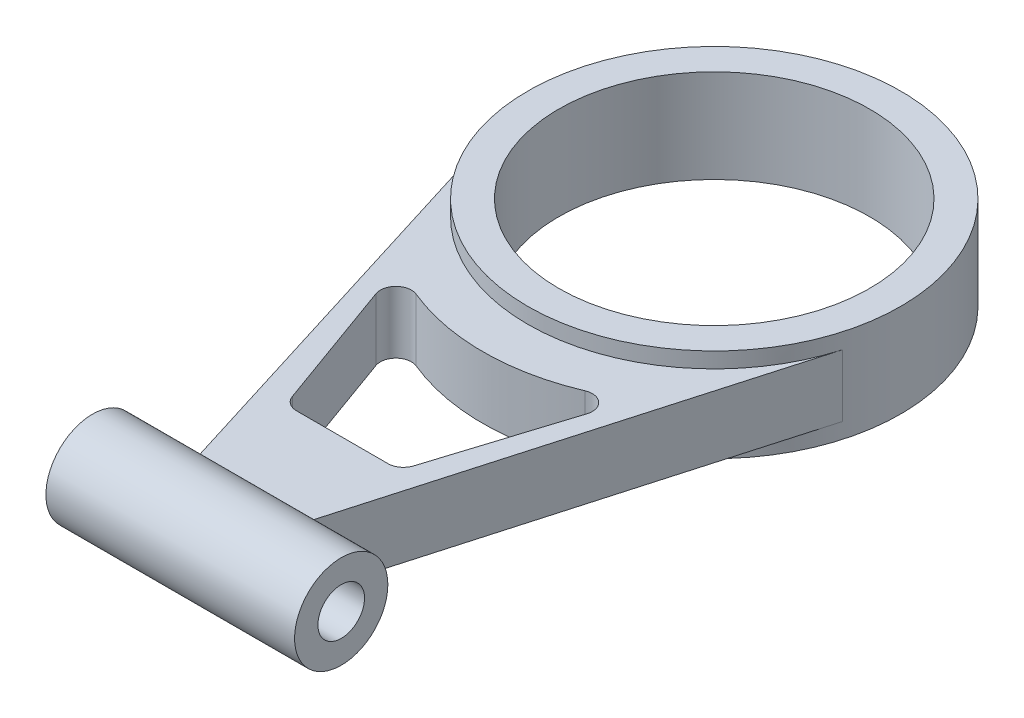
ISO-10303-21;
HEADER;
FILE_DESCRIPTION(('STEP AP214'),'2;1');
FILE_NAME('part.step','',(''),(''),'','','');
FILE_SCHEMA(('AUTOMOTIVE_DESIGN { 1 0 10303 214 1 1 1 1 }'));
ENDSEC;
DATA;
#1=APPLICATION_CONTEXT('core data for automotive mechanical design processes');
#2=APPLICATION_PROTOCOL_DEFINITION('international standard','automotive_design',2000,#1);
#3=PRODUCT_CONTEXT('',#1,'mechanical');
#4=PRODUCT('Part','Part','',(#3));
#5=PRODUCT_RELATED_PRODUCT_CATEGORY('part','',(#4));
#6=PRODUCT_DEFINITION_FORMATION('','',#4);
#7=PRODUCT_DEFINITION_CONTEXT('part definition',#1,'design');
#8=PRODUCT_DEFINITION('design','',#6,#7);
#9=PRODUCT_DEFINITION_SHAPE('','',#8);
#10=(LENGTH_UNIT() NAMED_UNIT(*) SI_UNIT(.MILLI.,.METRE.));
#11=(NAMED_UNIT(*) PLANE_ANGLE_UNIT() SI_UNIT($,.RADIAN.));
#12=(NAMED_UNIT(*) SI_UNIT($,.STERADIAN.) SOLID_ANGLE_UNIT());
#13=UNCERTAINTY_MEASURE_WITH_UNIT(LENGTH_MEASURE(1.E-05),#10,'distance_accuracy_value','');
#14=(GEOMETRIC_REPRESENTATION_CONTEXT(3) GLOBAL_UNCERTAINTY_ASSIGNED_CONTEXT((#13)) GLOBAL_UNIT_ASSIGNED_CONTEXT((#10,
#11,#12)) REPRESENTATION_CONTEXT('',''));
#15=CARTESIAN_POINT('',(0.,0.,0.));
#16=DIRECTION('',(0.,0.,1.));
#17=DIRECTION('',(1.,0.,0.));
#18=AXIS2_PLACEMENT_3D('',#15,#16,#17);
#19=CARTESIAN_POINT('',(40.,0.,0.));
#20=DIRECTION('',(1.,0.,0.));
#21=DIRECTION('',(0.,0.,-1.));
#22=AXIS2_PLACEMENT_3D('',#19,#20,#21);
#23=PLANE('',#22);
#24=CARTESIAN_POINT('',(40.,0.,0.));
#25=DIRECTION('',(1.,0.,0.));
#26=DIRECTION('',(0.,0.,-1.));
#27=AXIS2_PLACEMENT_3D('',#24,#25,#26);
#28=CIRCLE('',#27,15.);
#29=CARTESIAN_POINT('',(40.,0.,-15.));
#30=VERTEX_POINT('',#29);
#31=EDGE_CURVE('E219',#30,#30,#28,.T.);
#32=ORIENTED_EDGE('',*,*,#31,.T.);
#33=EDGE_LOOP('',(#32));
#34=FACE_BOUND('',#33,.T.);
#35=CARTESIAN_POINT('',(40.,0.,0.));
#36=DIRECTION('',(1.,0.,0.));
#37=DIRECTION('',(0.,0.,-1.));
#38=AXIS2_PLACEMENT_3D('',#35,#36,#37);
#39=CIRCLE('',#38,7.5);
#40=CARTESIAN_POINT('',(40.,0.,-7.5));
#41=VERTEX_POINT('',#40);
#42=EDGE_CURVE('E212',#41,#41,#39,.T.);
#43=ORIENTED_EDGE('',*,*,#42,.F.);
#44=EDGE_LOOP('',(#43));
#45=FACE_BOUND('',#44,.T.);
#46=ADVANCED_FACE('F43',(#34,#45),#23,.T.);
#47=CARTESIAN_POINT('',(-40.,0.,0.));
#48=DIRECTION('',(1.,0.,0.));
#49=DIRECTION('',(0.,0.,-1.));
#50=AXIS2_PLACEMENT_3D('',#47,#48,#49);
#51=PLANE('',#50);
#52=CARTESIAN_POINT('',(-40.,0.,0.));
#53=DIRECTION('',(1.,0.,0.));
#54=DIRECTION('',(0.,0.,-1.));
#55=AXIS2_PLACEMENT_3D('',#52,#53,#54);
#56=CIRCLE('',#55,15.);
#57=CARTESIAN_POINT('',(-40.,0.,-15.));
#58=VERTEX_POINT('',#57);
#59=EDGE_CURVE('E220',#58,#58,#56,.T.);
#60=ORIENTED_EDGE('',*,*,#59,.F.);
#61=EDGE_LOOP('',(#60));
#62=FACE_BOUND('',#61,.T.);
#63=CARTESIAN_POINT('',(-40.,0.,0.));
#64=DIRECTION('',(1.,0.,0.));
#65=DIRECTION('',(0.,0.,-1.));
#66=AXIS2_PLACEMENT_3D('',#63,#64,#65);
#67=CIRCLE('',#66,7.5);
#68=CARTESIAN_POINT('',(-40.,0.,-7.5));
#69=VERTEX_POINT('',#68);
#70=EDGE_CURVE('E213',#69,#69,#67,.T.);
#71=ORIENTED_EDGE('',*,*,#70,.T.);
#72=EDGE_LOOP('',(#71));
#73=FACE_BOUND('',#72,.T.);
#74=ADVANCED_FACE('F286',(#62,#73),#51,.F.);
#75=CARTESIAN_POINT('',(40.,0.,0.));
#76=DIRECTION('',(-1.,0.,0.));
#77=DIRECTION('',(0.,0.,1.));
#78=AXIS2_PLACEMENT_3D('',#75,#76,#77);
#79=CYLINDRICAL_SURFACE('',#78,15.);
#80=CARTESIAN_POINT('',(16.801488358698,0.,0.));
#81=DIRECTION('',(-0.961726920405214,0.,-0.274009727141033));
#82=DIRECTION('',(-0.274009727141033,0.,0.961726920405214));
#83=AXIS2_PLACEMENT_3D('',#80,#81,#82);
#84=ELLIPSE('',#83,15.596943042501,15.);
#85=CARTESIAN_POINT('',(19.986926778813,10.,-11.1803398874989));
#86=VERTEX_POINT('',#85);
#87=CARTESIAN_POINT('',(19.986926778813,-10.,-11.1803398874989));
#88=VERTEX_POINT('',#87);
#89=EDGE_CURVE('E226',#86,#88,#84,.T.);
#90=ORIENTED_EDGE('',*,*,#89,.F.);
#91=DIRECTION('',(-1.,0.,0.));
#92=VECTOR('',#91,1.);
#93=CARTESIAN_POINT('',(40.,10.,-11.1803398874989));
#94=LINE('',#93,#92);
#95=CARTESIAN_POINT('',(-16.5703284007776,10.,-11.1803398874989));
#96=VERTEX_POINT('',#95);
#97=EDGE_CURVE('E233',#86,#96,#94,.T.);
#98=ORIENTED_EDGE('',*,*,#97,.T.);
#99=CARTESIAN_POINT('',(-13.0948278450043,0.,0.));
#100=DIRECTION('',(-0.9549252516487,0.,0.29684636390508));
#101=DIRECTION('',(-0.29684636390508,0.,-0.9549252516487));
#102=AXIS2_PLACEMENT_3D('',#99,#100,#101);
#103=ELLIPSE('',#102,15.7080357589269,15.);
#104=CARTESIAN_POINT('',(-16.5703284007776,-10.,-11.1803398874989));
#105=VERTEX_POINT('',#104);
#106=EDGE_CURVE('E231',#96,#105,#103,.T.);
#107=ORIENTED_EDGE('',*,*,#106,.T.);
#108=DIRECTION('',(-1.,0.,0.));
#109=VECTOR('',#108,1.);
#110=CARTESIAN_POINT('',(40.,-10.,-11.1803398874989));
#111=LINE('',#110,#109);
#112=EDGE_CURVE('E224',#88,#105,#111,.T.);
#113=ORIENTED_EDGE('',*,*,#112,.F.);
#114=EDGE_LOOP('',(#90,#98,#107,#113));
#115=FACE_BOUND('',#114,.T.);
#116=ORIENTED_EDGE('',*,*,#31,.F.);
#117=EDGE_LOOP('',(#116));
#118=FACE_BOUND('',#117,.T.);
#119=ORIENTED_EDGE('',*,*,#59,.T.);
#120=EDGE_LOOP('',(#119));
#121=FACE_BOUND('',#120,.T.);
#122=ADVANCED_FACE('F44',(#115,#118,#121),#79,.T.);
#123=CARTESIAN_POINT('',(40.,0.,0.));
#124=DIRECTION('',(-1.,0.,0.));
#125=DIRECTION('',(0.,0.,1.));
#126=AXIS2_PLACEMENT_3D('',#123,#124,#125);
#127=CYLINDRICAL_SURFACE('',#126,7.5);
#128=ORIENTED_EDGE('',*,*,#42,.T.);
#129=EDGE_LOOP('',(#128));
#130=FACE_BOUND('',#129,.T.);
#131=ORIENTED_EDGE('',*,*,#70,.F.);
#132=EDGE_LOOP('',(#131));
#133=FACE_BOUND('',#132,.T.);
#134=ADVANCED_FACE('F293',(#130,#133),#127,.F.);
#135=CARTESIAN_POINT('',(0.,10.,0.));
#136=DIRECTION('',(0.,1.,0.));
#137=DIRECTION('',(0.,0.,1.));
#138=AXIS2_PLACEMENT_3D('',#135,#136,#137);
#139=PLANE('',#138);
#140=CARTESIAN_POINT('',(-13.0584068998663,10.,-43.7136049203832));
#141=DIRECTION('',(0.,1.,0.));
#142=DIRECTION('',(0.,0.,-1.));
#143=AXIS2_PLACEMENT_3D('',#140,#141,#142);
#144=CIRCLE('',#143,5.);
#145=CARTESIAN_POINT('',(-17.7618405284644,10.,-42.0172228580598));
#146=VERTEX_POINT('',#145);
#147=CARTESIAN_POINT('',(-13.0584068998663,10.,-38.7136049203832));
#148=VERTEX_POINT('',#147);
#149=EDGE_CURVE('E59',#146,#148,#144,.T.);
#150=ORIENTED_EDGE('',*,*,#149,.F.);
#151=DIRECTION('',(0.339276412464669,0.,0.940686725719622));
#152=VECTOR('',#151,1.);
#153=CARTESIAN_POINT('',(-32.9546293939201,10.,-84.1411498017971));
#154=LINE('',#153,#152);
#155=CARTESIAN_POINT('',(-32.9546293939206,10.,-84.1411498017969));
#156=VERTEX_POINT('',#155);
#157=EDGE_CURVE('E167',#156,#146,#154,.T.);
#158=ORIENTED_EDGE('',*,*,#157,.F.);
#159=CARTESIAN_POINT('',(-28.2511957653232,10.,-85.8375318641209));
#160=DIRECTION('',(0.,1.,0.));
#161=DIRECTION('',(0.,0.,1.));
#162=AXIS2_PLACEMENT_3D('',#159,#160,#161);
#163=CIRCLE('',#162,4.99999999999952);
#164=CARTESIAN_POINT('',(-26.341109619655,10.,-90.4583078721229));
#165=VERTEX_POINT('',#164);
#166=EDGE_CURVE('E162',#165,#156,#163,.T.);
#167=ORIENTED_EDGE('',*,*,#166,.F.);
#168=CARTESIAN_POINT('',(0.400096419681878,10.,-155.149171984157));
#169=DIRECTION('',(0.,-1.,0.));
#170=DIRECTION('',(0.,0.,1.));
#171=AXIS2_PLACEMENT_3D('',#168,#169,#170);
#172=CIRCLE('',#171,70.);
#173=CARTESIAN_POINT('',(27.7252493420679,10.,-90.702791032484));
#174=VERTEX_POINT('',#173);
#175=EDGE_CURVE('E159',#174,#165,#172,.T.);
#176=ORIENTED_EDGE('',*,*,#175,.F.);
#177=CARTESIAN_POINT('',(29.6770459793811,10.,-86.0994781073645));
#178=DIRECTION('',(0.,1.,0.));
#179=DIRECTION('',(0.,0.,1.));
#180=AXIS2_PLACEMENT_3D('',#177,#178,#179);
#181=CIRCLE('',#180,5.);
#182=CARTESIAN_POINT('',(34.4458674515617,10.,-84.5967000909994));
#183=VERTEX_POINT('',#182);
#184=EDGE_CURVE('E152',#183,#174,#181,.T.);
#185=ORIENTED_EDGE('',*,*,#184,.F.);
#186=DIRECTION('',(0.300555603273013,0.,-0.953764294436102));
#187=VECTOR('',#186,1.);
#188=CARTESIAN_POINT('',(21.088991166422,10.,-42.2108269040181));
#189=LINE('',#188,#187);
#190=CARTESIAN_POINT('',(21.088991166422,10.,-42.2108269040181));
#191=VERTEX_POINT('',#190);
#192=EDGE_CURVE('E155',#191,#183,#189,.T.);
#193=ORIENTED_EDGE('',*,*,#192,.F.);
#194=CARTESIAN_POINT('',(16.3201696942414,10.,-43.7136049203832));
#195=DIRECTION('',(0.,1.,0.));
#196=DIRECTION('',(0.,0.,1.));
#197=AXIS2_PLACEMENT_3D('',#194,#195,#196);
#198=CIRCLE('',#197,5.);
#199=CARTESIAN_POINT('',(16.3201696942414,10.,-38.7136049203832));
#200=VERTEX_POINT('',#199);
#201=EDGE_CURVE('E134',#200,#191,#198,.T.);
#202=ORIENTED_EDGE('',*,*,#201,.F.);
#203=DIRECTION('',(1.,0.,0.));
#204=VECTOR('',#203,1.);
#205=CARTESIAN_POINT('',(-13.0584068998663,10.,-38.7136049203832));
#206=LINE('',#205,#204);
#207=EDGE_CURVE('E145',#148,#200,#206,.T.);
#208=ORIENTED_EDGE('',*,*,#207,.F.);
#209=EDGE_LOOP('',(#150,#158,#167,#176,#185,#193,#202,#208));
#210=FACE_BOUND('',#209,.T.);
#211=ORIENTED_EDGE('',*,*,#97,.F.);
#212=DIRECTION('',(0.274009727141033,0.,-0.961726920405214));
#213=VECTOR('',#212,1.);
#214=CARTESIAN_POINT('',(15.5400102572058,10.,4.42757073759744));
#215=LINE('',#214,#213);
#216=CARTESIAN_POINT('',(57.7036152243128,10.,-143.559416371538));
#217=VERTEX_POINT('',#216);
#218=EDGE_CURVE('E199',#86,#217,#215,.T.);
#219=ORIENTED_EDGE('',*,*,#218,.T.);
#220=CARTESIAN_POINT('',(0.,10.,-160.));
#221=DIRECTION('',(0.,1.,0.));
#222=DIRECTION('',(0.,0.,1.));
#223=AXIS2_PLACEMENT_3D('',#220,#221,#222);
#224=CIRCLE('',#223,60.);
#225=CARTESIAN_POINT('',(-57.295515098922,10.,-142.189218165695));
#226=VERTEX_POINT('',#225);
#227=EDGE_CURVE('E192',#226,#217,#224,.T.);
#228=ORIENTED_EDGE('',*,*,#227,.F.);
#229=DIRECTION('',(-0.29684636390508,0.,-0.9549252516487));
#230=VECTOR('',#229,1.);
#231=CARTESIAN_POINT('',(-11.9409408984323,10.,3.71193963211804));
#232=LINE('',#231,#230);
#233=EDGE_CURVE('E197',#96,#226,#232,.T.);
#234=ORIENTED_EDGE('',*,*,#233,.F.);
#235=EDGE_LOOP('',(#211,#219,#228,#234));
#236=FACE_BOUND('',#235,.T.);
#237=ADVANCED_FACE('F146',(#210,#236),#139,.T.);
#238=CARTESIAN_POINT('',(0.,-10.,0.));
#239=DIRECTION('',(0.,1.,0.));
#240=DIRECTION('',(0.,0.,1.));
#241=AXIS2_PLACEMENT_3D('',#238,#239,#240);
#242=PLANE('',#241);
#243=DIRECTION('',(0.339276412464669,0.,0.940686725719622));
#244=VECTOR('',#243,1.);
#245=CARTESIAN_POINT('',(-2.30738693020975,-10.,0.832202622239151));
#246=LINE('',#245,#244);
#247=CARTESIAN_POINT('',(-32.9546293939206,-10.,-84.1411498017969));
#248=VERTEX_POINT('',#247);
#249=CARTESIAN_POINT('',(-17.7618405284644,-10.,-42.0172228580598));
#250=VERTEX_POINT('',#249);
#251=EDGE_CURVE('E51',#248,#250,#246,.T.);
#252=ORIENTED_EDGE('',*,*,#251,.T.);
#253=CARTESIAN_POINT('',(-13.0584068998663,-10.,-43.7136049203832));
#254=DIRECTION('',(0.,1.,0.));
#255=DIRECTION('',(0.,0.,1.));
#256=AXIS2_PLACEMENT_3D('',#253,#254,#255);
#257=CIRCLE('',#256,5.);
#258=CARTESIAN_POINT('',(-13.0584068998663,-10.,-38.7136049203832));
#259=VERTEX_POINT('',#258);
#260=EDGE_CURVE('E11',#250,#259,#257,.T.);
#261=ORIENTED_EDGE('',*,*,#260,.T.);
#262=DIRECTION('',(1.,0.,0.));
#263=VECTOR('',#262,1.);
#264=CARTESIAN_POINT('',(0.,-10.,-38.7136049203832));
#265=LINE('',#264,#263);
#266=CARTESIAN_POINT('',(16.3201696942414,-10.,-38.7136049203832));
#267=VERTEX_POINT('',#266);
#268=EDGE_CURVE('E234',#259,#267,#265,.T.);
#269=ORIENTED_EDGE('',*,*,#268,.T.);
#270=CARTESIAN_POINT('',(16.3201696942414,-10.,-43.7136049203832));
#271=DIRECTION('',(0.,1.,0.));
#272=DIRECTION('',(0.,0.,1.));
#273=AXIS2_PLACEMENT_3D('',#270,#271,#272);
#274=CIRCLE('',#273,5.);
#275=CARTESIAN_POINT('',(21.088991166422,-10.,-42.2108269040181));
#276=VERTEX_POINT('',#275);
#277=EDGE_CURVE('E138',#267,#276,#274,.T.);
#278=ORIENTED_EDGE('',*,*,#277,.T.);
#279=DIRECTION('',(0.300555603273013,0.,-0.953764294436102));
#280=VECTOR('',#279,1.);
#281=CARTESIAN_POINT('',(7.08382319004432,-10.,2.23229446183233));
#282=LINE('',#281,#280);
#283=CARTESIAN_POINT('',(34.4458674515617,-10.,-84.5967000909994));
#284=VERTEX_POINT('',#283);
#285=EDGE_CURVE('E236',#276,#284,#282,.T.);
#286=ORIENTED_EDGE('',*,*,#285,.T.);
#287=CARTESIAN_POINT('',(29.6770459793811,-10.,-86.0994781073645));
#288=DIRECTION('',(0.,1.,0.));
#289=DIRECTION('',(0.,0.,1.));
#290=AXIS2_PLACEMENT_3D('',#287,#288,#289);
#291=CIRCLE('',#290,5.);
#292=CARTESIAN_POINT('',(27.7252493420679,-10.,-90.702791032484));
#293=VERTEX_POINT('',#292);
#294=EDGE_CURVE('E243',#284,#293,#291,.T.);
#295=ORIENTED_EDGE('',*,*,#294,.T.);
#296=CARTESIAN_POINT('',(0.400096419681878,-10.,-155.149171984157));
#297=DIRECTION('',(0.,1.,0.));
#298=DIRECTION('',(0.,0.,1.));
#299=AXIS2_PLACEMENT_3D('',#296,#297,#298);
#300=CIRCLE('',#299,70.);
#301=CARTESIAN_POINT('',(-26.341109619655,-10.,-90.4583078721229));
#302=VERTEX_POINT('',#301);
#303=EDGE_CURVE('E242',#293,#302,#300,.F.);
#304=ORIENTED_EDGE('',*,*,#303,.T.);
#305=CARTESIAN_POINT('',(-28.2511957653232,-10.,-85.8375318641209));
#306=DIRECTION('',(0.,1.,0.));
#307=DIRECTION('',(0.,0.,1.));
#308=AXIS2_PLACEMENT_3D('',#305,#306,#307);
#309=CIRCLE('',#308,4.99999999999952);
#310=EDGE_CURVE('E250',#302,#248,#309,.T.);
#311=ORIENTED_EDGE('',*,*,#310,.T.);
#312=EDGE_LOOP('',(#252,#261,#269,#278,#286,#295,#304,#311));
#313=FACE_BOUND('',#312,.T.);
#314=DIRECTION('',(0.274009727141033,0.,-0.961726920405214));
#315=VECTOR('',#314,1.);
#316=CARTESIAN_POINT('',(15.5400102572058,-10.,4.42757073759744));
#317=LINE('',#316,#315);
#318=CARTESIAN_POINT('',(57.7036152243128,-10.,-143.559416371538));
#319=VERTEX_POINT('',#318);
#320=EDGE_CURVE('E196',#88,#319,#317,.T.);
#321=ORIENTED_EDGE('',*,*,#320,.F.);
#322=ORIENTED_EDGE('',*,*,#112,.T.);
#323=DIRECTION('',(-0.29684636390508,0.,-0.9549252516487));
#324=VECTOR('',#323,1.);
#325=CARTESIAN_POINT('',(-11.9409408984323,-10.,3.71193963211804));
#326=LINE('',#325,#324);
#327=CARTESIAN_POINT('',(-57.295515098922,-10.,-142.189218165695));
#328=VERTEX_POINT('',#327);
#329=EDGE_CURVE('E204',#105,#328,#326,.T.);
#330=ORIENTED_EDGE('',*,*,#329,.T.);
#331=CARTESIAN_POINT('',(0.,-10.,-160.));
#332=DIRECTION('',(0.,1.,0.));
#333=DIRECTION('',(0.,0.,1.));
#334=AXIS2_PLACEMENT_3D('',#331,#332,#333);
#335=CIRCLE('',#334,60.);
#336=EDGE_CURVE('E191',#328,#319,#335,.T.);
#337=ORIENTED_EDGE('',*,*,#336,.T.);
#338=EDGE_LOOP('',(#321,#322,#330,#337));
#339=FACE_BOUND('',#338,.T.);
#340=ADVANCED_FACE('F253',(#313,#339),#242,.F.);
#341=CARTESIAN_POINT('',(-11.9409408984323,10.,3.71193963211804));
#342=DIRECTION('',(-0.9549252516487,0.,0.29684636390508));
#343=DIRECTION('',(0.29684636390508,0.,0.9549252516487));
#344=AXIS2_PLACEMENT_3D('',#341,#342,#343);
#345=PLANE('',#344);
#346=ORIENTED_EDGE('',*,*,#106,.F.);
#347=ORIENTED_EDGE('',*,*,#233,.T.);
#348=DIRECTION('',(0.,-1.,0.));
#349=VECTOR('',#348,1.);
#350=CARTESIAN_POINT('',(-57.295515098922,10.,-142.189218165695));
#351=LINE('',#350,#349);
#352=EDGE_CURVE('E209',#226,#328,#351,.T.);
#353=ORIENTED_EDGE('',*,*,#352,.T.);
#354=ORIENTED_EDGE('',*,*,#329,.F.);
#355=EDGE_LOOP('',(#346,#347,#353,#354));
#356=FACE_BOUND('',#355,.T.);
#357=ADVANCED_FACE('F297',(#356),#345,.T.);
#358=CARTESIAN_POINT('',(15.5400102572058,10.,4.42757073759744));
#359=DIRECTION('',(-0.961726920405214,0.,-0.274009727141033));
#360=DIRECTION('',(-0.274009727141033,0.,0.961726920405214));
#361=AXIS2_PLACEMENT_3D('',#358,#359,#360);
#362=PLANE('',#361);
#363=ORIENTED_EDGE('',*,*,#218,.F.);
#364=ORIENTED_EDGE('',*,*,#89,.T.);
#365=ORIENTED_EDGE('',*,*,#320,.T.);
#366=DIRECTION('',(0.,-1.,0.));
#367=VECTOR('',#366,1.);
#368=CARTESIAN_POINT('',(57.7036152243128,10.,-143.559416371538));
#369=LINE('',#368,#367);
#370=EDGE_CURVE('E205',#217,#319,#369,.T.);
#371=ORIENTED_EDGE('',*,*,#370,.F.);
#372=EDGE_LOOP('',(#363,#364,#365,#371));
#373=FACE_BOUND('',#372,.T.);
#374=ADVANCED_FACE('F305',(#373),#362,.F.);
#375=CARTESIAN_POINT('',(0.,15.,-160.));
#376=DIRECTION('',(0.,-1.,0.));
#377=DIRECTION('',(0.,0.,-1.));
#378=AXIS2_PLACEMENT_3D('',#375,#376,#377);
#379=CYLINDRICAL_SURFACE('',#378,60.);
#380=CARTESIAN_POINT('',(0.,15.,-160.));
#381=DIRECTION('',(0.,1.,0.));
#382=DIRECTION('',(0.,0.,1.));
#383=AXIS2_PLACEMENT_3D('',#380,#381,#382);
#384=CIRCLE('',#383,60.);
#385=CARTESIAN_POINT('',(0.,15.,-100.));
#386=VERTEX_POINT('',#385);
#387=EDGE_CURVE('E186',#386,#386,#384,.T.);
#388=ORIENTED_EDGE('',*,*,#387,.F.);
#389=EDGE_LOOP('',(#388));
#390=FACE_BOUND('',#389,.T.);
#391=CARTESIAN_POINT('',(0.,-15.,-160.));
#392=DIRECTION('',(0.,1.,0.));
#393=DIRECTION('',(0.,0.,1.));
#394=AXIS2_PLACEMENT_3D('',#391,#392,#393);
#395=CIRCLE('',#394,60.);
#396=CARTESIAN_POINT('',(0.,-15.,-100.));
#397=VERTEX_POINT('',#396);
#398=EDGE_CURVE('E183',#397,#397,#395,.T.);
#399=ORIENTED_EDGE('',*,*,#398,.T.);
#400=EDGE_LOOP('',(#399));
#401=FACE_BOUND('',#400,.T.);
#402=ORIENTED_EDGE('',*,*,#336,.F.);
#403=ORIENTED_EDGE('',*,*,#352,.F.);
#404=ORIENTED_EDGE('',*,*,#227,.T.);
#405=ORIENTED_EDGE('',*,*,#370,.T.);
#406=EDGE_LOOP('',(#402,#403,#404,#405));
#407=FACE_BOUND('',#406,.T.);
#408=ADVANCED_FACE('F308',(#390,#401,#407),#379,.T.);
#409=CARTESIAN_POINT('',(0.,15.,-160.));
#410=DIRECTION('',(0.,1.,0.));
#411=DIRECTION('',(0.,0.,1.));
#412=AXIS2_PLACEMENT_3D('',#409,#410,#411);
#413=PLANE('',#412);
#414=ORIENTED_EDGE('',*,*,#387,.T.);
#415=EDGE_LOOP('',(#414));
#416=FACE_BOUND('',#415,.T.);
#417=CARTESIAN_POINT('',(0.,15.,-160.));
#418=DIRECTION('',(0.,1.,0.));
#419=DIRECTION('',(0.,0.,1.));
#420=AXIS2_PLACEMENT_3D('',#417,#418,#419);
#421=CIRCLE('',#420,50.);
#422=CARTESIAN_POINT('',(0.,15.,-110.));
#423=VERTEX_POINT('',#422);
#424=EDGE_CURVE('E185',#423,#423,#421,.T.);
#425=ORIENTED_EDGE('',*,*,#424,.F.);
#426=EDGE_LOOP('',(#425));
#427=FACE_BOUND('',#426,.T.);
#428=ADVANCED_FACE('F311',(#416,#427),#413,.T.);
#429=CARTESIAN_POINT('',(0.,-15.,-160.));
#430=DIRECTION('',(0.,1.,0.));
#431=DIRECTION('',(0.,0.,1.));
#432=AXIS2_PLACEMENT_3D('',#429,#430,#431);
#433=PLANE('',#432);
#434=ORIENTED_EDGE('',*,*,#398,.F.);
#435=EDGE_LOOP('',(#434));
#436=FACE_BOUND('',#435,.T.);
#437=CARTESIAN_POINT('',(0.,-15.,-160.));
#438=DIRECTION('',(0.,1.,0.));
#439=DIRECTION('',(0.,0.,1.));
#440=AXIS2_PLACEMENT_3D('',#437,#438,#439);
#441=CIRCLE('',#440,50.);
#442=CARTESIAN_POINT('',(0.,-15.,-110.));
#443=VERTEX_POINT('',#442);
#444=EDGE_CURVE('E173',#443,#443,#441,.T.);
#445=ORIENTED_EDGE('',*,*,#444,.T.);
#446=EDGE_LOOP('',(#445));
#447=FACE_BOUND('',#446,.T.);
#448=ADVANCED_FACE('F283',(#436,#447),#433,.F.);
#449=CARTESIAN_POINT('',(0.,15.,-160.));
#450=DIRECTION('',(0.,-1.,0.));
#451=DIRECTION('',(0.,0.,-1.));
#452=AXIS2_PLACEMENT_3D('',#449,#450,#451);
#453=CYLINDRICAL_SURFACE('',#452,50.);
#454=ORIENTED_EDGE('',*,*,#424,.T.);
#455=EDGE_LOOP('',(#454));
#456=FACE_BOUND('',#455,.T.);
#457=ORIENTED_EDGE('',*,*,#444,.F.);
#458=EDGE_LOOP('',(#457));
#459=FACE_BOUND('',#458,.T.);
#460=ADVANCED_FACE('F272',(#456,#459),#453,.F.);
#461=CARTESIAN_POINT('',(-13.0584068998663,-15.,-43.7136049203832));
#462=DIRECTION('',(0.,1.,0.));
#463=DIRECTION('',(0.,0.,1.));
#464=AXIS2_PLACEMENT_3D('',#461,#462,#463);
#465=CYLINDRICAL_SURFACE('',#464,5.);
#466=DIRECTION('',(0.,1.,0.));
#467=VECTOR('',#466,1.);
#468=CARTESIAN_POINT('',(-17.7618405284644,-15.,-42.0172228580598));
#469=LINE('',#468,#467);
#470=EDGE_CURVE('E166',#250,#146,#469,.T.);
#471=ORIENTED_EDGE('',*,*,#470,.T.);
#472=ORIENTED_EDGE('',*,*,#149,.T.);
#473=DIRECTION('',(0.,1.,0.));
#474=VECTOR('',#473,1.);
#475=CARTESIAN_POINT('',(-13.0584068998663,-15.,-38.7136049203832));
#476=LINE('',#475,#474);
#477=EDGE_CURVE('E143',#259,#148,#476,.T.);
#478=ORIENTED_EDGE('',*,*,#477,.F.);
#479=ORIENTED_EDGE('',*,*,#260,.F.);
#480=EDGE_LOOP('',(#471,#472,#478,#479));
#481=FACE_BOUND('',#480,.T.);
#482=ADVANCED_FACE('F271',(#481),#465,.F.);
#483=CARTESIAN_POINT('',(-32.9546293939201,-15.,-84.1411498017971));
#484=DIRECTION('',(-0.940686725719622,0.,0.339276412464669));
#485=DIRECTION('',(0.339276412464669,0.,0.940686725719622));
#486=AXIS2_PLACEMENT_3D('',#483,#484,#485);
#487=PLANE('',#486);
#488=DIRECTION('',(0.,1.,0.));
#489=VECTOR('',#488,1.);
#490=CARTESIAN_POINT('',(-32.9546293939206,-15.,-84.1411498017969));
#491=LINE('',#490,#489);
#492=EDGE_CURVE('E175',#248,#156,#491,.T.);
#493=ORIENTED_EDGE('',*,*,#492,.T.);
#494=ORIENTED_EDGE('',*,*,#157,.T.);
#495=ORIENTED_EDGE('',*,*,#470,.F.);
#496=ORIENTED_EDGE('',*,*,#251,.F.);
#497=EDGE_LOOP('',(#493,#494,#495,#496));
#498=FACE_BOUND('',#497,.T.);
#499=ADVANCED_FACE('F258',(#498),#487,.F.);
#500=CARTESIAN_POINT('',(-28.2511957653232,-15.,-85.8375318641209));
#501=DIRECTION('',(0.,1.,0.));
#502=DIRECTION('',(0.,0.,1.));
#503=AXIS2_PLACEMENT_3D('',#500,#501,#502);
#504=CYLINDRICAL_SURFACE('',#503,4.99999999999952);
#505=DIRECTION('',(0.,1.,0.));
#506=VECTOR('',#505,1.);
#507=CARTESIAN_POINT('',(-26.341109619655,-15.,-90.4583078721229));
#508=LINE('',#507,#506);
#509=EDGE_CURVE('E172',#302,#165,#508,.T.);
#510=ORIENTED_EDGE('',*,*,#509,.T.);
#511=ORIENTED_EDGE('',*,*,#166,.T.);
#512=ORIENTED_EDGE('',*,*,#492,.F.);
#513=ORIENTED_EDGE('',*,*,#310,.F.);
#514=EDGE_LOOP('',(#510,#511,#512,#513));
#515=FACE_BOUND('',#514,.T.);
#516=ADVANCED_FACE('F256',(#515),#504,.F.);
#517=CARTESIAN_POINT('',(0.400096419681878,-15.,-155.149171984157));
#518=DIRECTION('',(0.,1.,0.));
#519=DIRECTION('',(0.,0.,1.));
#520=AXIS2_PLACEMENT_3D('',#517,#518,#519);
#521=CYLINDRICAL_SURFACE('',#520,70.);
#522=DIRECTION('',(0.,1.,0.));
#523=VECTOR('',#522,1.);
#524=CARTESIAN_POINT('',(27.7252493420679,-15.,-90.702791032484));
#525=LINE('',#524,#523);
#526=EDGE_CURVE('E176',#293,#174,#525,.T.);
#527=ORIENTED_EDGE('',*,*,#526,.T.);
#528=ORIENTED_EDGE('',*,*,#175,.T.);
#529=ORIENTED_EDGE('',*,*,#509,.F.);
#530=ORIENTED_EDGE('',*,*,#303,.F.);
#531=EDGE_LOOP('',(#527,#528,#529,#530));
#532=FACE_BOUND('',#531,.T.);
#533=ADVANCED_FACE('F262',(#532),#521,.T.);
#534=CARTESIAN_POINT('',(29.6770459793811,-15.,-86.0994781073645));
#535=DIRECTION('',(0.,1.,0.));
#536=DIRECTION('',(0.,0.,1.));
#537=AXIS2_PLACEMENT_3D('',#534,#535,#536);
#538=CYLINDRICAL_SURFACE('',#537,5.);
#539=DIRECTION('',(0.,1.,0.));
#540=VECTOR('',#539,1.);
#541=CARTESIAN_POINT('',(34.4458674515617,-15.,-84.5967000909994));
#542=LINE('',#541,#540);
#543=EDGE_CURVE('E178',#284,#183,#542,.T.);
#544=ORIENTED_EDGE('',*,*,#543,.T.);
#545=ORIENTED_EDGE('',*,*,#184,.T.);
#546=ORIENTED_EDGE('',*,*,#526,.F.);
#547=ORIENTED_EDGE('',*,*,#294,.F.);
#548=EDGE_LOOP('',(#544,#545,#546,#547));
#549=FACE_BOUND('',#548,.T.);
#550=ADVANCED_FACE('F270',(#549),#538,.F.);
#551=CARTESIAN_POINT('',(21.088991166422,-15.,-42.2108269040181));
#552=DIRECTION('',(0.953764294436102,0.,0.300555603273013));
#553=DIRECTION('',(0.300555603273013,0.,-0.953764294436102));
#554=AXIS2_PLACEMENT_3D('',#551,#552,#553);
#555=PLANE('',#554);
#556=DIRECTION('',(0.,1.,0.));
#557=VECTOR('',#556,1.);
#558=CARTESIAN_POINT('',(21.088991166422,-15.,-42.2108269040181));
#559=LINE('',#558,#557);
#560=EDGE_CURVE('E139',#276,#191,#559,.T.);
#561=ORIENTED_EDGE('',*,*,#560,.T.);
#562=ORIENTED_EDGE('',*,*,#192,.T.);
#563=ORIENTED_EDGE('',*,*,#543,.F.);
#564=ORIENTED_EDGE('',*,*,#285,.F.);
#565=EDGE_LOOP('',(#561,#562,#563,#564));
#566=FACE_BOUND('',#565,.T.);
#567=ADVANCED_FACE('F269',(#566),#555,.F.);
#568=CARTESIAN_POINT('',(16.3201696942414,-15.,-43.7136049203832));
#569=DIRECTION('',(0.,1.,0.));
#570=DIRECTION('',(0.,0.,1.));
#571=AXIS2_PLACEMENT_3D('',#568,#569,#570);
#572=CYLINDRICAL_SURFACE('',#571,5.);
#573=DIRECTION('',(0.,1.,0.));
#574=VECTOR('',#573,1.);
#575=CARTESIAN_POINT('',(16.3201696942414,-15.,-38.7136049203832));
#576=LINE('',#575,#574);
#577=EDGE_CURVE('E66',#267,#200,#576,.T.);
#578=ORIENTED_EDGE('',*,*,#577,.T.);
#579=ORIENTED_EDGE('',*,*,#201,.T.);
#580=ORIENTED_EDGE('',*,*,#560,.F.);
#581=ORIENTED_EDGE('',*,*,#277,.F.);
#582=EDGE_LOOP('',(#578,#579,#580,#581));
#583=FACE_BOUND('',#582,.T.);
#584=ADVANCED_FACE('F135',(#583),#572,.F.);
#585=CARTESIAN_POINT('',(-13.0584068998663,-15.,-38.7136049203832));
#586=DIRECTION('',(0.,0.,1.));
#587=DIRECTION('',(1.,0.,0.));
#588=AXIS2_PLACEMENT_3D('',#585,#586,#587);
#589=PLANE('',#588);
#590=ORIENTED_EDGE('',*,*,#477,.T.);
#591=ORIENTED_EDGE('',*,*,#207,.T.);
#592=ORIENTED_EDGE('',*,*,#577,.F.);
#593=ORIENTED_EDGE('',*,*,#268,.F.);
#594=EDGE_LOOP('',(#590,#591,#592,#593));
#595=FACE_BOUND('',#594,.T.);
#596=ADVANCED_FACE('F144',(#595),#589,.F.);
#597=CLOSED_SHELL('',(#46,#74,#122,#134,#237,#340,#357,#374,#408,#428,#448,#460,#482,#499,#516,
#533,#550,#567,#584,#596));
#598=MANIFOLD_SOLID_BREP('B2',#597);
#599=ADVANCED_BREP_SHAPE_REPRESENTATION('',(#18,#598),#14);
#600=SHAPE_DEFINITION_REPRESENTATION(#9,#599);
ENDSEC;
END-ISO-10303-21;
